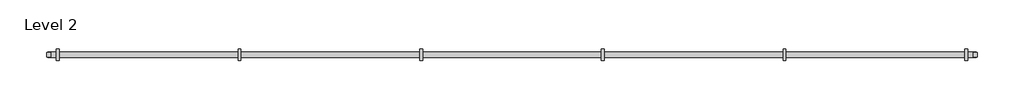
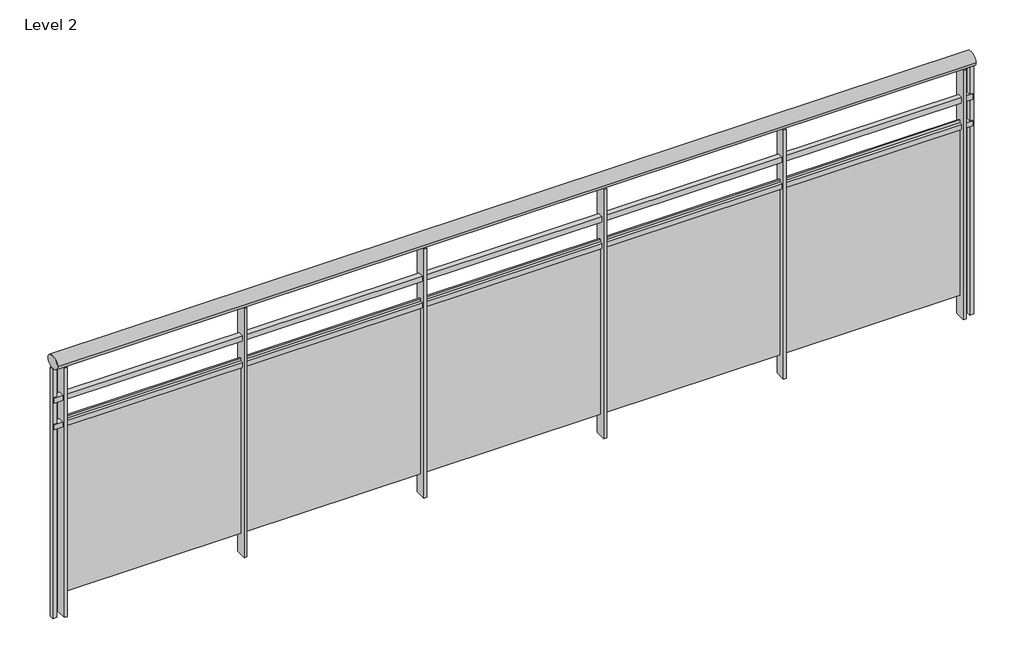
# One storey: 1 railing.
"""IFC4 building model written with IfcOpenShell, lengths in millimetres."""

from ifc_helpers import new_model, si_unit, point, frame, origin, place, context, project, spatial, polyline, ellipse_curve, trimmed, outline, extrude, element, save
from ifc_brep_helpers import plane_surface, extruded_surface, advanced_brep

model = new_model("IFC4")

# Units and contexts
model_context = context("Model", 3, world=origin())
ifc_project = project(units=[si_unit("LENGTHUNIT", "METRE", prefix="MILLI")], contexts=[model_context])

# Site, building, storey
site = spatial("IfcSite", under=ifc_project)
building = spatial("IfcBuilding", under=site)
storey = spatial("IfcBuildingStorey", under=building, Name="Level 2", Elevation=3200.4)

# Railing
placement = place(None, origin())
element("IfcRailing", 1, ObjectType="Glass Panel - Bottom Fill", at=placement, inside=storey, context=model_context, shape_type="SolidModel", body=[
    advanced_brep(
    [(-5729.1673724, -5829.5544725, 4419.6), (-5729.1673724, -5905.7544725, 4419.6), (-1576.8982041, -5829.5544725, 4419.6), (-1576.8982041, -5905.7544725, 4419.6)],
    [
        (0, 1, ellipse_curve(frame((-5729.1673724, -5867.6544725, 4419.6), z_axis=(-1.0, 0.0, 0.0), x_axis=(0.0, -1.0, 0.0)), 38.1, 28.575)),
        (1, 0, ellipse_curve(frame((-5729.1673724, -5867.6544725, 4419.6), z_axis=(-1.0, 0.0, 0.0), x_axis=(0.0, -1.0, 0.0)), 38.1, 28.575)),
        (2, 3, ellipse_curve(frame((-1576.8982041, -5867.6544725, 4419.6), z_axis=(1.0, 0.0, 0.0), x_axis=(0.0, -1.0, 0.0)), 38.1, 28.575)),
        (3, 2, ellipse_curve(frame((-1576.8982041, -5867.6544725, 4419.6), z_axis=(1.0, 0.0, 0.0), x_axis=(0.0, -1.0, 0.0)), 38.1, 28.575)),
        (0, 2),
        (3, 1),
    ],
    [
        plane_surface(frame((-5729.1673724, -5867.6544725, 4419.6), z_axis=(-1.0, 0.0, 0.0), x_axis=(0.0, 1.0, 0.0))),
        plane_surface(frame((-1576.8982041, -5867.6544725, 4419.6), z_axis=(1.0, 0.0, 0.0), x_axis=(0.0, 1.0, 0.0))),
        extruded_surface(trimmed(ellipse_curve(frame((-1576.8982041, -5867.6544725, 4419.6), z_axis=(-1.0, 0.0, 0.0), x_axis=(0.0, -1.0, 0.0)), 38.1, 28.575), [point((-1576.8982041, -5829.5544725, 4419.6))], [point((-1576.8982041, -5905.7544725, 4419.6))], True, "CARTESIAN"), (-4152.2691683, 0.0, 0.0), 4152.2691683),
        extruded_surface(trimmed(ellipse_curve(frame((-1576.8982041, -5867.6544725, 4419.6), z_axis=(-1.0, 0.0, 0.0), x_axis=(0.0, -1.0, 0.0)), 38.1, 28.575), [point((-1576.8982041, -5905.7544725, 4419.6))], [point((-1576.8982041, -5829.5544725, 4419.6))], True, "CARTESIAN"), (-4152.2691683, 0.0, 0.0), 4152.2691683),
    ],
    [
        (0, [[1, 2]]),
        (1, [[3, 4]]),
        (2, [[-1, 5, -4, 6]]),
        (3, [[-2, -6, -3, -5]]),
    ],
),
    extrude(outline(polyline([(-5729.1673724, -5880.3544725), (-5729.1673724, -5854.9544725), (-1576.8982041, -5854.9544725), (-1576.8982041, -5880.3544725), (-5729.1673724, -5880.3544725)])), frame((0.0, 0.0, 4229.1), z_axis=(0.0, 0.0, 1.0), x_axis=(1.0, 0.0, 0.0)), (0.0, 0.0, 1.0), 25.4),
    extrude(outline(polyline([(-5729.1673724, -5880.3544725), (-5729.1673724, -5854.9544725), (-1576.8982041, -5854.9544725), (-1576.8982041, -5880.3544725), (-5729.1673724, -5880.3544725)])), frame((0.0, 0.0, 4102.1), z_axis=(0.0, 0.0, 1.0), x_axis=(1.0, 0.0, 0.0)), (0.0, 0.0, 1.0), 25.4),
    extrude(outline(polyline([(-1627.3827882, -5893.0544725), (-1627.3827882, -5842.2544725), (-1614.6827882, -5842.2544725), (-1614.6827882, -5893.0544725), (-1627.3827882, -5893.0544725)])), frame((0.0, 0.0, 3200.4), z_axis=(0.0, 0.0, 1.0), x_axis=(1.0, 0.0, 0.0)), (0.0, 0.0, 1.0), 1190.625),
    extrude(outline(polyline([(-2433.8327882, -5861.1193155), (-1621.0327882, -5861.1193155), (-1621.0327882, -5867.4693155), (-2433.8327882, -5867.4693155), (-2433.8327882, -5861.1193155)])), frame((0.0, 0.0, 3302.0), z_axis=(0.0, 0.0, 1.0), x_axis=(1.0, 0.0, 0.0)), (0.0, 0.0, 1.0), 838.2),
    extrude(outline(polyline([(-2440.1827882, -5893.0544725), (-2440.1827882, -5842.2544725), (-2427.4827882, -5842.2544725), (-2427.4827882, -5893.0544725), (-2440.1827882, -5893.0544725)])), frame((0.0, 0.0, 3200.4), z_axis=(0.0, 0.0, 1.0), x_axis=(1.0, 0.0, 0.0)), (0.0, 0.0, 1.0), 1190.625),
    extrude(outline(polyline([(-3246.6327882, -5861.1193155), (-2433.8327882, -5861.1193155), (-2433.8327882, -5867.4693155), (-3246.6327882, -5867.4693155), (-3246.6327882, -5861.1193155)])), frame((0.0, 0.0, 3302.0), z_axis=(0.0, 0.0, 1.0), x_axis=(1.0, 0.0, 0.0)), (0.0, 0.0, 1.0), 838.2),
    extrude(outline(polyline([(-3252.9827882, -5893.0544725), (-3252.9827882, -5842.2544725), (-3240.2827882, -5842.2544725), (-3240.2827882, -5893.0544725), (-3252.9827882, -5893.0544725)])), frame((0.0, 0.0, 3200.4), z_axis=(0.0, 0.0, 1.0), x_axis=(1.0, 0.0, 0.0)), (0.0, 0.0, 1.0), 1190.625),
    extrude(outline(polyline([(-4059.4327882, -5861.1193155), (-3246.6327882, -5861.1193155), (-3246.6327882, -5867.4693155), (-4059.4327882, -5867.4693155), (-4059.4327882, -5861.1193155)])), frame((0.0, 0.0, 3302.0), z_axis=(0.0, 0.0, 1.0), x_axis=(1.0, 0.0, 0.0)), (0.0, 0.0, 1.0), 838.2),
    extrude(outline(polyline([(-4065.7827882, -5893.0544725), (-4065.7827882, -5842.2544725), (-4053.0827882, -5842.2544725), (-4053.0827882, -5893.0544725), (-4065.7827882, -5893.0544725)])), frame((0.0, 0.0, 3200.4), z_axis=(0.0, 0.0, 1.0), x_axis=(1.0, 0.0, 0.0)), (0.0, 0.0, 1.0), 1190.625),
    extrude(outline(polyline([(-4872.2327882, -5861.1193155), (-4059.4327882, -5861.1193155), (-4059.4327882, -5867.4693155), (-4872.2327882, -5867.4693155), (-4872.2327882, -5861.1193155)])), frame((0.0, 0.0, 3302.0), z_axis=(0.0, 0.0, 1.0), x_axis=(1.0, 0.0, 0.0)), (0.0, 0.0, 1.0), 838.2),
    extrude(outline(polyline([(-4878.5827882, -5893.0544725), (-4878.5827882, -5842.2544725), (-4865.8827882, -5842.2544725), (-4865.8827882, -5893.0544725), (-4878.5827882, -5893.0544725)])), frame((0.0, 0.0, 3200.4), z_axis=(0.0, 0.0, 1.0), x_axis=(1.0, 0.0, 0.0)), (0.0, 0.0, 1.0), 1190.625),
    extrude(outline(polyline([(-5685.0327882, -5861.1193155), (-4872.2327882, -5861.1193155), (-4872.2327882, -5867.4693155), (-5685.0327882, -5867.4693155), (-5685.0327882, -5861.1193155)])), frame((0.0, 0.0, 3302.0), z_axis=(0.0, 0.0, 1.0), x_axis=(1.0, 0.0, 0.0)), (0.0, 0.0, 1.0), 838.2),
    extrude(outline(polyline([(-5691.3827882, -5893.0544725), (-5691.3827882, -5842.2544725), (-5678.6827882, -5842.2544725), (-5678.6827882, -5893.0544725), (-5691.3827882, -5893.0544725)])), frame((0.0, 0.0, 3200.4), z_axis=(0.0, 0.0, 1.0), x_axis=(1.0, 0.0, 0.0)), (0.0, 0.0, 1.0), 1190.625),
    extrude(outline(polyline([(-1589.5982041, -5877.1794725), (-1589.5982041, -5858.1294725), (-1570.5482041, -5858.1294725), (-1570.5482041, -5877.1794725), (-1589.5982041, -5877.1794725)])), frame((0.0, 0.0, 3200.4), z_axis=(0.0, 0.0, 1.0), x_axis=(1.0, 0.0, 0.0)), (0.0, 0.0, 1.0), 1190.625),
    extrude(outline(polyline([(-5735.5173724, -5877.1794725), (-5735.5173724, -5858.1294725), (-5716.4673724, -5858.1294725), (-5716.4673724, -5877.1794725), (-5735.5173724, -5877.1794725)])), frame((0.0, 0.0, 3200.4), z_axis=(0.0, 0.0, 1.0), x_axis=(1.0, 0.0, 0.0)), (0.0, 0.0, 1.0), 1190.625),
])

save(model, "model.ifc")

# Revit data of these elements
# Type "Glass Panel - Bottom Fill"
#   Assembly Code = "C2010400"
#   built-in parameter 1008612 = 0.0416667 (stored number, unit not read)
#   built-in parameter 1008611 = 0.0416667 (stored number, unit not read)
#   built-in parameter 1008609 = 0.333333 (stored number, unit not read)
#   built-in parameter 1008604 = 0.166667 (stored number, unit not read)
#   built-in parameter 1008603 = 0.166667 (stored number, unit not read)
#   Railing Height = 4' - 0"
#   built-in parameter 1008630 = 2
#   built-in parameter 1008610 = 2
#   built-in parameter 1008618 = Baluster - Square : 3/4"
# Element 1 (IfcRailing, "Glass Panel - Bottom Fill")
#   Phase Created = New Construction
#   Materials on its faces: "Glass"
# Materials
#   "Glass": class "Glass", colour RGB 0 128 192, transparency 0.75, Description = "Soda Lime Glass", Cost = 0
